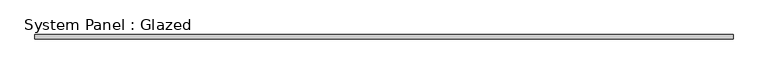
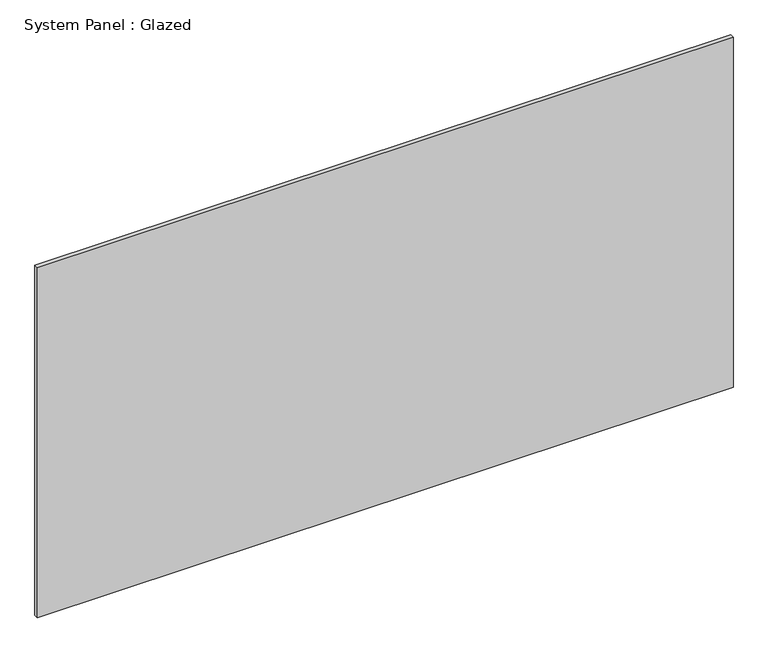
"""IFC4 building model written with IfcOpenShell, lengths in millimetres: plate geometry, System Panel : Glazed."""

from ifc_helpers import new_model, si_unit, origin, origin_with_axes, place, context, project, spatial, polyline, outline, extrude, source, transform, mapped, element, save


def system_panel_glazed_c41ca4f4(model_context):
    return source(origin(), model_context, "Body", "SweptSolid", [
        extrude(outline(polyline([(2006.6, 19.05), (-2006.6, 19.05), (-2006.6, 44.45), (2006.6, 44.45), (2006.6, 19.05)])), origin_with_axes(), (0.0, 0.0, 1.0), 2133.6),
    ])


if __name__ == "__main__":
    model = new_model("IFC4")
    model_context = context("Model", 3, world=origin())
    ifc_project = project(units=[si_unit("LENGTHUNIT", "METRE", prefix="MILLI")], contexts=[model_context])
    site = spatial("IfcSite", under=ifc_project)
    building = spatial("IfcBuilding", under=site)
    placement = place(None, origin())
    system_panel_glazed_shape = system_panel_glazed_c41ca4f4(model_context)
    element("IfcPlate", 1, ObjectType="System Panel : Glazed", at=placement, inside=building, context=model_context, shape_type="MappedRepresentation", body=[
        mapped(system_panel_glazed_shape, transform((0.0, 0.0, 0.0), x_axis=(1.0, 0.0, 0.0), y_axis=(0.0, 1.0, 0.0), z_axis=(0.0, 0.0, 1.0))),
    ])
    save(model, "model.ifc")

# Revit data of these elements
# Type "System Panel : Glazed"
#   Construction Type Id = "GSP4R"
#   Analytic Construction = "1/8 in Pilkington single glazing"
#   Visual Light Transmittance = 0.9
#   Solar Heat Gain Coefficient = 0.86
#   Heat Transfer Coefficient (U) = 1.18115 BTU/(h·ft²·°F)
# Element 1 (IfcPlate, "System Panel : Glazed")
#   Materials on its faces: "Glass"
# Materials
#   "Glass": class "Glass", colour RGB 0 128 192, transparency 0.75, Description = "Soda Lime Glass", Cost = 0
